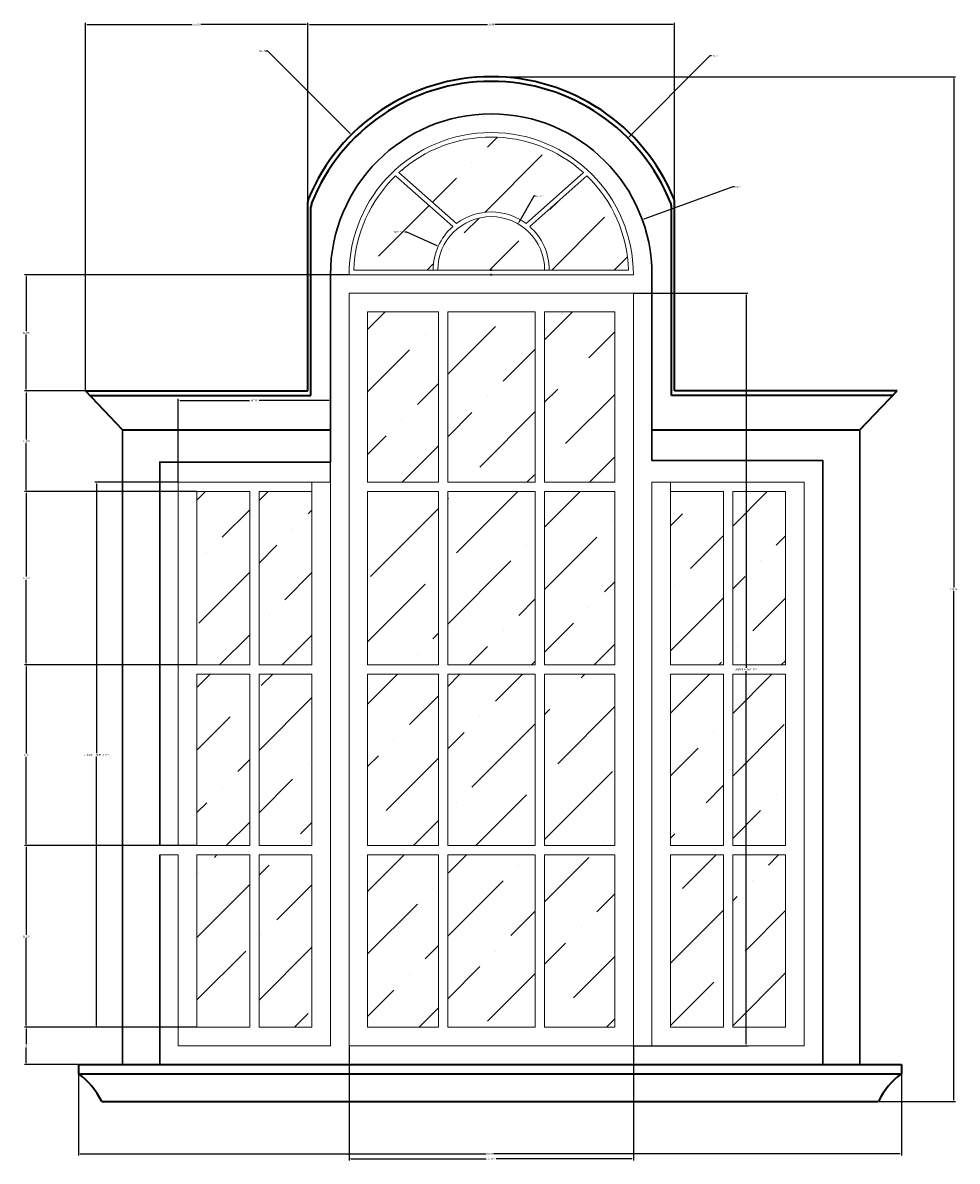
# Model space of a CAD drawing. Units: inches. Extents: x 386 to 708, y 151 to 489.
# Tile 1 of 4: x 386 to 486, y 159 to 281. Entities that reach past the tile are written whole.
import ezdxf

# ---------------------------------------------------------------- set-up
doc = ezdxf.new("R2010")
doc.units = ezdxf.units.IN
doc.header["$MEASUREMENT"] = 0
for name, color, linetype, lineweight in [('A-ANNO-DIMS', 2, 'Continuous', 18), ('A-GLAZ-FRAM', 4, 'Continuous', 30), ('A-GLAZ-PATT', 252, 'Continuous', 13), ('A-GLAZ-SASH', 4, 'Continuous', 18), ('A-GLAZ-SILL', 7, 'Continuous', 35), ('A-GLAZ-TRIM', 7, 'Continuous', 35)]:
    doc.layers.add(name, color=color, linetype=linetype, lineweight=lineweight)
doc.styles.get("Standard").update_dxf_attribs({"font": 'arial.ttf'})
doc.dimstyles.get("Standard").update_dxf_attribs({"dimtxt": 0.18, "dimasz": 0.18, "dimexe": 0.18, "dimexo": 0.0625, "dimgap": 0.09, "dimtad": 0, "dimtih": 1, "dimtoh": 1, "dimdec": 4, "dimzin": 0, "dimdsep": 46, "dimtxsty": 'Standard', "dimcen": 0.09, "dimadec": 0, "dimazin": 0, "dimtfac": 1, "dimtdec": 4, "dimtofl": 0, "dimtmove": 0, "dimatfit": 3, "dimfxl": 1, "dimtolj": 1, "dimtzin": 0, "dimarcsym": 0})

# ---------------------------------------------------------------- blocks, each defined once
blk = doc.blocks.new('WIN-SASH-3X4')
for p, q in [((9.62, 60.63), (9.62, 78.96)), ((10.62, 60.63), (10.62, 78.96)), ((20.04, 60.63), (20.04, 78.96)), ((21.04, 60.63), (21.04, 78.96)), ((2, 60.63), (9.62, 60.63)), ((10.62, 60.63), (20.04, 60.63)), ((21.04, 60.63), (28.6, 60.63)), ((21.04, 60.63), (28.6, 60.63)), ((2, 59.63), (9.62, 59.63)), ((9.62, 40.98), (9.62, 59.63)), ((10.62, 40.98), (10.62, 59.63)), ((10.62, 59.63), (20.04, 59.63)), ((20.04, 40.98), (20.04, 59.63)), ((21.04, 59.63), (28.6, 59.63)), ((21.04, 40.98), (21.04, 59.63)), ((21.04, 59.63), (28.6, 59.63)), ((2, 40.98), (9.62, 40.98)), ((10.62, 40.98), (20.04, 40.98)), ((21.04, 40.98), (28.6, 40.98)), ((21.04, 40.98), (28.6, 40.98)), ((2, 39.98), (9.62, 39.98)), ((9.62, 21.54), (9.62, 39.98)), ((10.62, 21.54), (10.62, 39.98)), ((10.62, 39.98), (20.04, 39.98)), ((20.04, 21.54), (20.04, 39.98)), ((21.04, 39.98), (28.6, 39.98)), ((21.04, 21.54), (21.04, 39.98)), ((21.04, 39.98), (28.6, 39.98)), ((2, 21.54), (9.62, 21.54)), ((10.62, 21.54), (20.04, 21.54)), ((21.04, 21.54), (28.6, 21.54)), ((21.04, 21.54), (28.6, 21.54)), ((2, 20.54), (9.62, 20.54)), ((9.62, 2), (9.62, 20.54)), ((10.62, 2), (10.62, 20.54)), ((10.62, 20.54), (20.04, 20.54)), ((20.04, 2), (20.04, 20.54)), ((21.04, 2), (21.04, 20.54)), ((21.04, 20.54), (28.6, 20.54)), ((21.04, 20.54), (28.6, 20.54))]:
    blk.add_line(p, q)
blk.add_lwpolyline([(30.6, 0), (30.6, 80.96), (0, 80.96), (0, 0)], close=True)
for points in [[(9.62, 78.96), (2, 78.96), (2, 60.63)], [(20.04, 78.96), (10.62, 78.96)], [(28.6, 60.63), (28.6, 78.96), (21.04, 78.96)], [(2, 59.63), (2, 40.98)], [(28.6, 40.98), (28.6, 59.63)], [(2, 39.98), (2, 21.54)], [(28.6, 21.54), (28.6, 39.98)], [(2, 20.54), (2, 2), (9.62, 2)], [(21.04, 2), (28.6, 2), (28.6, 20.54)], [(10.62, 2), (20.04, 2)]]:
    blk.add_lwpolyline(points)
blk = doc.blocks.new('WIN-FANLIGHT-RADIAL')
for p, q in [((11.16, 5.18), (5.01, 10.63)), ((11.55, 5.5), (5.37, 10.98)), ((19.05, 5.5), (25.23, 10.98)), ((19.44, 5.18), (25.6, 10.63))]:
    blk.add_line(p, q)
blk.add_lwpolyline([(30.6, 0), (0, 0, -1)], format="xyb", close=True)
for points in [[(5.37, 10.98, -0.385138), (25.23, 10.98, -0.385138)], [(25.6, 10.63, -0.194348), (30.09, 0.5), (0.51, 0.5, -0.194348), (5.01, 10.63)]]:
    blk.add_lwpolyline(points, format="xyb")
for radius, start, end in [(5.75, 0, 180), (6.25, 53.1161, 126.8839), (6.25, 131.5309, 180), (6.25, 0, 48.4691)]:
    blk.add_arc((15.3, 0.5), radius, start, end)
blk = doc.blocks.new('WIN-SILL-TRIPLE')
for p, q in [((0, 4), (88.59, 4)), ((0, 4), (0, 3)), ((88.59, 4), (88.59, 3)), ((0, 3), (88.59, 3)), ((2.5, 0), (86.09, 0))]:
    blk.add_line(p, q)
blk.add_lwpolyline([(4.75, 0), (84.1, 0)])
for centre, start, end in [((-4.74, -3.48), 25.6893, 53.8074), ((93.33, -3.48), 126.1926, 154.3107)]:
    blk.add_arc(centre, 8.03, start, end)
blk = doc.blocks.new('WIN-LIGHT-GRID-2X3')
for p, q in [((0, 58.63), (7.69, 58.63)), ((2, 57.63), (7.69, 57.63)), ((7.69, 58.63), (16.38, 58.63)), ((7.69, 38.98), (7.69, 57.63)), ((8.69, 38.98), (8.69, 57.63)), ((8.69, 57.63), (14.38, 57.63)), ((2, 38.98), (7.69, 38.98)), ((2, 37.98), (7.69, 37.98)), ((7.69, 19.54), (7.69, 37.98)), ((8.69, 38.98), (14.38, 38.98)), ((8.69, 19.54), (8.69, 37.98)), ((8.69, 37.98), (14.38, 37.98)), ((2, 19.54), (7.69, 19.54)), ((2, 18.54), (7.69, 18.54)), ((7.69, 0), (7.69, 18.54)), ((8.69, 19.54), (14.38, 19.54)), ((8.69, 0), (8.69, 18.54)), ((8.69, 18.54), (14.38, 18.54))]:
    blk.add_line(p, q)
for points in [[(2, 57.63), (2, 38.98)], [(14.38, 38.98), (14.38, 58.63)], [(2, 37.98), (2, 19.54)], [(14.38, 19.54), (14.38, 37.98)], [(2, 18.54), (2, 0), (7.69, 0)], [(8.69, 0), (14.38, 0), (14.38, 18.54)]]:
    blk.add_lwpolyline(points)
blk = doc.blocks.new('*D12')
at = {"layer": 'A-ANNO-DIMS', "color": 0, "lineweight": -2, "transparency": 16777216}
for p, q in [((451.56, 252.21), (463.82, 252.21)), ((463.64, 252.03), (463.64, 211.91)), ((463.64, 171.43), (463.64, 211.55)), ((451.56, 171.25), (463.82, 171.25))]:
    blk.add_line(p, q, dxfattribs=at)
at = {"layer": 'A-ANNO-DIMS', "color": 0, "transparency": 16777216}
for points in [[(463.61, 252.03), (463.67, 252.03), (463.64, 252.21)], [(463.61, 171.43), (463.67, 171.43), (463.64, 171.25)]]:
    blk.add_solid(points, dxfattribs=at)
at = {"layer": 'Defpoints', "color": 0, "transparency": 16777216}
for p in [(451.5, 252.21), (463.64, 252.21), (451.5, 171.25)]:
    blk.add_point(p, dxfattribs=at)
at = {"layer": 'A-ANNO-DIMS', "color": 0, "transparency": 16777216, "insert": (463.64, 211.73), "char_height": 0.18, "attachment_point": 5}
blk.add_mtext('\\A1;CENTRE SASH 81 TYP.', dxfattribs=at)
blk = doc.blocks.new('*D13')
at = {"layer": 'A-ANNO-DIMS', "color": 0, "lineweight": -2, "transparency": 16777216}
for p, q in [((420.9, 171.19), (420.9, 158.93)), ((451.5, 171.19), (451.5, 158.93)), ((421.08, 159.11), (435.67, 159.11)), ((451.32, 159.11), (436.73, 159.11))]:
    blk.add_line(p, q, dxfattribs=at)
at = {"layer": 'A-ANNO-DIMS', "color": 0, "transparency": 16777216}
for points in [[(421.08, 159.14), (421.08, 159.08), (420.9, 159.11)], [(451.32, 159.14), (451.32, 159.08), (451.5, 159.11)]]:
    blk.add_solid(points, dxfattribs=at)
at = {"layer": 'Defpoints', "color": 0, "transparency": 16777216}
for p in [(420.9, 171.25), (451.5, 171.25), (451.5, 159.11)]:
    blk.add_point(p, dxfattribs=at)
at = {"layer": 'A-ANNO-DIMS', "color": 0, "transparency": 16777216, "insert": (436.2, 159.11), "char_height": 0.18, "attachment_point": 5}
blk.add_mtext('\\A1;31 TYP.', dxfattribs=at)
blk = doc.blocks.new('*D20')
at = {"layer": 'A-ANNO-DIMS', "color": 0, "lineweight": -2, "transparency": 16777216}
for p, q in [((402.46, 231.88), (393.55, 231.88)), ((393.73, 231.7), (393.73, 202.75)), ((393.73, 173.43), (393.73, 202.38)), ((402.46, 173.25), (393.55, 173.25))]:
    blk.add_line(p, q, dxfattribs=at)
at = {"layer": 'A-ANNO-DIMS', "color": 0, "transparency": 16777216}
for points in [[(393.7, 231.7), (393.76, 231.7), (393.73, 231.88)], [(393.7, 173.43), (393.76, 173.43), (393.73, 173.25)]]:
    blk.add_solid(points, dxfattribs=at)
at = {"layer": 'Defpoints', "color": 0, "transparency": 16777216}
for p in [(393.73, 231.88), (402.52, 231.88), (402.52, 173.25)]:
    blk.add_point(p, dxfattribs=at)
at = {"layer": 'A-ANNO-DIMS', "color": 0, "transparency": 16777216, "insert": (393.73, 202.57), "char_height": 0.18, "attachment_point": 5}
blk.add_mtext('\\A1;SIDELIGHT GRID 59 TYP.', dxfattribs=at)
blk = doc.blocks.new('*D21')
at = {"layer": 'A-ANNO-DIMS', "color": 0, "lineweight": -2, "transparency": 16777216}
for p, q in [((402.52, 231.94), (402.52, 240.85)), ((402.7, 240.67), (410.19, 240.67)), ((418.72, 240.67), (411.23, 240.67)), ((418.9, 231.94), (418.9, 240.85))]:
    blk.add_line(p, q, dxfattribs=at)
at = {"layer": 'A-ANNO-DIMS', "color": 0, "transparency": 16777216}
for points in [[(402.7, 240.7), (402.7, 240.64), (402.52, 240.67)], [(418.72, 240.7), (418.72, 240.64), (418.9, 240.67)]]:
    blk.add_solid(points, dxfattribs=at)
at = {"layer": 'Defpoints', "color": 0, "transparency": 16777216}
for p in [(418.9, 240.67), (402.52, 231.88), (418.9, 231.88)]:
    blk.add_point(p, dxfattribs=at)
at = {"layer": 'A-ANNO-DIMS', "color": 0, "transparency": 16777216, "insert": (410.71, 240.67), "char_height": 0.18, "attachment_point": 5}
blk.add_mtext('\\A1;16 TYP.', dxfattribs=at)
blk = doc.blocks.new('*D35')
at = {"layer": 'A-ANNO-DIMS', "color": 0, "lineweight": -2, "transparency": 16777216}
for p, q in [((391.77, 169.19), (391.77, 159.45)), ((480.36, 169.19), (480.36, 159.45)), ((391.95, 159.63), (435.67, 159.63)), ((480.18, 159.63), (436.46, 159.63))]:
    blk.add_line(p, q, dxfattribs=at)
at = {"layer": 'A-ANNO-DIMS', "color": 0, "transparency": 16777216}
for points in [[(391.95, 159.66), (391.95, 159.6), (391.77, 159.63)], [(480.18, 159.66), (480.18, 159.6), (480.36, 159.63)]]:
    blk.add_solid(points, dxfattribs=at)
at = {"layer": 'Defpoints', "color": 0, "transparency": 16777216}
for p in [(391.77, 169.25), (480.36, 169.25), (480.36, 159.63)]:
    blk.add_point(p, dxfattribs=at)
at = {"layer": 'A-ANNO-DIMS', "color": 0, "transparency": 16777216, "insert": (436.07, 159.63), "char_height": 0.18, "attachment_point": 5}
blk.add_mtext('\\A1;88.59', dxfattribs=at)
blk = doc.blocks.new('*D36')
at = {"layer": 'A-ANNO-DIMS', "color": 0, "lineweight": -2, "transparency": 16777216}
for p, q in [((436.26, 275.51), (486.16, 275.51)), ((485.98, 275.33), (485.98, 220.56)), ((485.98, 165.43), (485.98, 220.2)), ((477.93, 165.25), (486.16, 165.25))]:
    blk.add_line(p, q, dxfattribs=at)
at = {"layer": 'A-ANNO-DIMS', "color": 0, "transparency": 16777216}
for points in [[(485.95, 275.33), (486.01, 275.33), (485.98, 275.51)], [(485.95, 165.43), (486.01, 165.43), (485.98, 165.25)]]:
    blk.add_solid(points, dxfattribs=at)
at = {"layer": 'Defpoints', "color": 0, "transparency": 16777216}
for p in [(436.2, 275.51), (485.98, 275.51), (477.87, 165.25)]:
    blk.add_point(p, dxfattribs=at)
at = {"layer": 'A-ANNO-DIMS', "color": 0, "transparency": 16777216, "insert": (485.98, 220.38), "char_height": 0.18, "attachment_point": 5}
blk.add_mtext('\\A1;110.26', dxfattribs=at)
blk = doc.blocks.new('*D37')
at = {"layer": 'A-ANNO-DIMS', "color": 0, "lineweight": -2, "transparency": 16777216}
for p, q in [((404.45689, 173.252448), (385.969656, 173.252448)), ((386.149656, 173.072448), (386.149656, 171.432448)), ((386.149656, 169.432448), (386.149656, 171.072448)), ((391.710656, 169.252448), (385.969656, 169.252448))]:
    blk.add_line(p, q, dxfattribs=at)
at = {"layer": 'A-ANNO-DIMS', "color": 0, "transparency": 16777216}
for points in [[(386.119656, 173.072448), (386.179656, 173.072448), (386.149656, 173.252448)], [(386.119656, 169.432448), (386.179656, 169.432448), (386.149656, 169.252448)]]:
    blk.add_solid(points, dxfattribs=at)
at = {"layer": 'Defpoints', "color": 0, "transparency": 16777216}
for p in [(386.149656, 173.252448), (404.51939, 173.252448), (391.773156, 169.252448)]:
    blk.add_point(p, dxfattribs=at)
at = {"layer": 'A-ANNO-DIMS', "color": 0, "transparency": 16777216, "insert": (386.149656, 171.252448), "char_height": 0.18, "attachment_point": 5}
blk.add_mtext('\\A1;4', dxfattribs=at)
blk = doc.blocks.new('*D38')
at = {"layer": 'A-ANNO-DIMS', "color": 0, "lineweight": -2, "transparency": 16777216}
for p, q in [((404.46, 192.79), (385.97, 192.79)), ((386.15, 192.61), (386.15, 183.2)), ((386.15, 173.43), (386.15, 182.84)), ((404.46, 173.25), (385.97, 173.25))]:
    blk.add_line(p, q, dxfattribs=at)
at = {"layer": 'A-ANNO-DIMS', "color": 0, "transparency": 16777216}
for points in [[(386.12, 192.61), (386.18, 192.61), (386.15, 192.79)], [(386.12, 173.43), (386.18, 173.43), (386.15, 173.25)]]:
    blk.add_solid(points, dxfattribs=at)
at = {"layer": 'Defpoints', "color": 0, "transparency": 16777216}
for p in [(386.15, 192.79), (404.52, 192.79), (404.52, 173.25)]:
    blk.add_point(p, dxfattribs=at)
at = {"layer": 'A-ANNO-DIMS', "color": 0, "transparency": 16777216, "insert": (386.15, 183.02), "char_height": 0.18, "attachment_point": 5}
blk.add_mtext('\\A1;19.537', dxfattribs=at)
blk = doc.blocks.new('*D39')
at = {"layer": 'A-ANNO-DIMS', "color": 0, "lineweight": -2, "transparency": 16777216}
for p, q in [((404.46, 212.23), (385.97, 212.23)), ((386.15, 212.05), (386.15, 202.69)), ((386.15, 192.97), (386.15, 202.33)), ((404.46, 192.79), (385.97, 192.79))]:
    blk.add_line(p, q, dxfattribs=at)
at = {"layer": 'A-ANNO-DIMS', "color": 0, "transparency": 16777216}
for points in [[(386.12, 212.05), (386.18, 212.05), (386.15, 212.23)], [(386.12, 192.97), (386.18, 192.97), (386.15, 192.79)]]:
    blk.add_solid(points, dxfattribs=at)
at = {"layer": 'Defpoints', "color": 0, "transparency": 16777216}
for p in [(386.15, 212.23), (404.52, 212.23), (404.52, 192.79)]:
    blk.add_point(p, dxfattribs=at)
at = {"layer": 'A-ANNO-DIMS', "color": 0, "transparency": 16777216, "insert": (386.15, 202.51), "char_height": 0.18, "attachment_point": 5}
blk.add_mtext('\\A1;19.44', dxfattribs=at)
blk = doc.blocks.new('*D40')
at = {"layer": 'A-ANNO-DIMS', "color": 0, "lineweight": -2, "transparency": 16777216}
for p, q in [((404.46, 230.88), (385.97, 230.88)), ((386.15, 230.7), (386.15, 221.74)), ((386.15, 212.41), (386.15, 221.37)), ((404.46, 212.23), (385.97, 212.23))]:
    blk.add_line(p, q, dxfattribs=at)
at = {"layer": 'A-ANNO-DIMS', "color": 0, "transparency": 16777216}
for points in [[(386.12, 230.7), (386.18, 230.7), (386.15, 230.88)], [(386.12, 212.41), (386.18, 212.41), (386.15, 212.23)]]:
    blk.add_solid(points, dxfattribs=at)
at = {"layer": 'Defpoints', "color": 0, "transparency": 16777216}
for p in [(386.15, 230.88), (404.52, 230.88), (404.52, 212.23)]:
    blk.add_point(p, dxfattribs=at)
at = {"layer": 'A-ANNO-DIMS', "color": 0, "transparency": 16777216, "insert": (386.15, 221.55), "char_height": 0.18, "attachment_point": 5}
blk.add_mtext('\\A1;18.648', dxfattribs=at)
blk = doc.blocks.new('*D41')
at = {"layer": 'A-ANNO-DIMS', "color": 0, "lineweight": -2, "transparency": 16777216}
for p, q in [((392.46, 241.7), (385.97, 241.7)), ((386.15, 241.52), (386.15, 236.47)), ((386.15, 231.06), (386.15, 236.11)), ((404.46, 230.88), (385.97, 230.88))]:
    blk.add_line(p, q, dxfattribs=at)
at = {"layer": 'A-ANNO-DIMS', "color": 0, "transparency": 16777216}
for points in [[(386.12, 241.52), (386.18, 241.52), (386.15, 241.7)], [(386.12, 231.06), (386.18, 231.06), (386.15, 230.88)]]:
    blk.add_solid(points, dxfattribs=at)
at = {"layer": 'Defpoints', "color": 0, "transparency": 16777216}
for p in [(386.15, 241.7), (392.52, 241.7), (404.52, 230.88)]:
    blk.add_point(p, dxfattribs=at)
at = {"layer": 'A-ANNO-DIMS', "color": 0, "transparency": 16777216, "insert": (386.15, 236.29), "char_height": 0.18, "attachment_point": 5}
blk.add_mtext('\\A1;10.825', dxfattribs=at)
blk = doc.blocks.new('*D42')
at = {"layer": 'A-ANNO-DIMS', "color": 0, "lineweight": -2, "transparency": 16777216}
for p, q in [((420.83, 254.21), (385.97, 254.21)), ((386.15, 254.03), (386.15, 248.14)), ((386.15, 241.88), (386.15, 247.77)), ((392.46, 241.7), (385.97, 241.7))]:
    blk.add_line(p, q, dxfattribs=at)
at = {"layer": 'A-ANNO-DIMS', "color": 0, "transparency": 16777216}
for points in [[(386.12, 254.03), (386.18, 254.03), (386.15, 254.21)], [(386.12, 241.88), (386.18, 241.88), (386.15, 241.7)]]:
    blk.add_solid(points, dxfattribs=at)
at = {"layer": 'Defpoints', "color": 0, "transparency": 16777216}
for p in [(386.15, 254.21), (420.9, 254.21), (392.52, 241.7)]:
    blk.add_point(p, dxfattribs=at)
at = {"layer": 'A-ANNO-DIMS', "color": 0, "transparency": 16777216, "insert": (386.15, 247.96), "char_height": 0.18, "attachment_point": 5}
blk.add_mtext('\\A1;12.505', dxfattribs=at)
blk = doc.blocks.new('*D43')
at = {"layer": 'A-ANNO-DIMS', "color": 0, "lineweight": -2, "transparency": 16777216}
for p, q in [((416.46, 241.77), (416.46, 281.31)), ((416.64, 281.13), (435.8, 281.13)), ((455.76, 281.13), (436.59, 281.13)), ((455.94, 241.77), (455.94, 281.31))]:
    blk.add_line(p, q, dxfattribs=at)
at = {"layer": 'A-ANNO-DIMS', "color": 0, "transparency": 16777216}
for points in [[(416.64, 281.16), (416.64, 281.1), (416.46, 281.13)], [(455.76, 281.16), (455.76, 281.1), (455.94, 281.13)]]:
    blk.add_solid(points, dxfattribs=at)
at = {"layer": 'Defpoints', "color": 0, "transparency": 16777216}
for p in [(455.94, 281.13), (416.46, 241.7), (455.94, 241.7)]:
    blk.add_point(p, dxfattribs=at)
at = {"layer": 'A-ANNO-DIMS', "color": 0, "transparency": 16777216, "insert": (436.2, 281.13), "char_height": 0.18, "attachment_point": 5}
blk.add_mtext('\\A1;39.48', dxfattribs=at)
blk = doc.blocks.new('*D44')
at = {"layer": 'A-ANNO-DIMS', "color": 0, "lineweight": -2, "transparency": 16777216}
for p, q in [((392.52, 241.77), (392.52, 281.31)), ((392.7, 281.13), (404.02, 281.13)), ((416.28, 281.13), (404.95, 281.13)), ((416.46, 241.77), (416.46, 281.31))]:
    blk.add_line(p, q, dxfattribs=at)
at = {"layer": 'A-ANNO-DIMS', "color": 0, "transparency": 16777216}
for points in [[(392.7, 281.16), (392.7, 281.1), (392.52, 281.13)], [(416.28, 281.16), (416.28, 281.1), (416.46, 281.13)]]:
    blk.add_solid(points, dxfattribs=at)
at = {"layer": 'Defpoints', "color": 0, "transparency": 16777216}
for p in [(416.46, 281.13), (392.52, 241.7), (416.46, 241.7)]:
    blk.add_point(p, dxfattribs=at)
at = {"layer": 'A-ANNO-DIMS', "color": 0, "transparency": 16777216, "insert": (404.49, 281.13), "char_height": 0.18, "attachment_point": 5}
blk.add_mtext('\\A1;23.937', dxfattribs=at)
blk = doc.blocks.new('*D83')
at = {"layer": 'A-ANNO-DIMS', "color": 0, "lineweight": -2, "transparency": 16777216}
for p, q in [((411.92, 278.31), (412.1, 278.31)), ((412.1, 278.31), (421.01, 269.4)), ((436.11, 254.21), (436.29, 254.21)), ((436.2, 254.12), (436.2, 254.3))]:
    blk.add_line(p, q, dxfattribs=at)
at = {"layer": 'A-ANNO-DIMS', "color": 0, "transparency": 16777216}
blk.add_solid([(421.03, 269.42), (420.99, 269.38), (421.14, 269.27)], dxfattribs=at)
at = {"layer": 'Defpoints', "color": 0, "transparency": 16777216}
for p in [(421.14, 269.27), (436.2, 254.21)]:
    blk.add_point(p, dxfattribs=at)
at = {"layer": 'A-ANNO-DIMS', "color": 0, "transparency": 16777216, "insert": (411.51, 278.31), "char_height": 0.18, "attachment_point": 5}
blk.add_mtext('\\A1;R21.3', dxfattribs=at)
blk = doc.blocks.new('*D84')
at = {"layer": 'A-ANNO-DIMS', "color": 0, "lineweight": -2, "transparency": 16777216}
for p, q in [((459.73, 277.74), (451.03, 269.04)), ((459.91, 277.74), (459.73, 277.74)), ((436.11, 254.21), (436.29, 254.21)), ((436.2, 254.12), (436.2, 254.3))]:
    blk.add_line(p, q, dxfattribs=at)
at = {"layer": 'A-ANNO-DIMS', "color": 0, "transparency": 16777216}
blk.add_solid([(451.01, 269.07), (451.06, 269.02), (450.91, 268.92)], dxfattribs=at)
at = {"layer": 'Defpoints', "color": 0, "transparency": 16777216}
for p in [(450.91, 268.92), (436.2, 254.21)]:
    blk.add_point(p, dxfattribs=at)
at = {"layer": 'A-ANNO-DIMS', "color": 0, "transparency": 16777216, "insert": (460.32, 277.74), "char_height": 0.18, "attachment_point": 5}
blk.add_mtext('\\A1;R20.8', dxfattribs=at)
blk = doc.blocks.new('*D85')
at = {"layer": 'A-ANNO-DIMS', "color": 0, "lineweight": -2, "transparency": 16777216}
for p, q in [((462.21, 263.68), (452.63, 260.19)), ((462.39, 263.68), (462.21, 263.68)), ((436.11, 254.21), (436.29, 254.21)), ((436.2, 254.12), (436.2, 254.3))]:
    blk.add_line(p, q, dxfattribs=at)
at = {"layer": 'A-ANNO-DIMS', "color": 0, "transparency": 16777216}
blk.add_solid([(452.62, 260.22), (452.64, 260.16), (452.46, 260.13)], dxfattribs=at)
at = {"layer": 'Defpoints', "color": 0, "transparency": 16777216}
for p in [(452.46, 260.13), (436.2, 254.21)]:
    blk.add_point(p, dxfattribs=at)
at = {"layer": 'A-ANNO-DIMS', "color": 0, "transparency": 16777216, "insert": (462.8, 263.68), "char_height": 0.18, "attachment_point": 5}
blk.add_mtext('\\A1;R17.3', dxfattribs=at)
blk = doc.blocks.new('*D86')
at = {"layer": 'A-ANNO-DIMS', "color": 0, "lineweight": -2, "transparency": 16777216}
for p, q in [((426.9, 258.81), (427.08, 258.81)), ((427.08, 258.81), (430.34, 257.35)), ((436.2, 254.62), (436.2, 254.8)), ((436.11, 254.71), (436.29, 254.71))]:
    blk.add_line(p, q, dxfattribs=at)
at = {"layer": 'A-ANNO-DIMS', "color": 0, "transparency": 16777216}
blk.add_solid([(430.35, 257.37), (430.33, 257.32), (430.5, 257.27)], dxfattribs=at)
at = {"layer": 'Defpoints', "color": 0, "transparency": 16777216}
for p in [(430.5, 257.27), (436.2, 254.71)]:
    blk.add_point(p, dxfattribs=at)
at = {"layer": 'A-ANNO-DIMS', "color": 0, "transparency": 16777216, "insert": (426.23, 258.81), "char_height": 0.18, "attachment_point": 5}
blk.add_mtext('\\A1;3X R6.247', dxfattribs=at)
blk = doc.blocks.new('*D87')
at = {"layer": 'A-ANNO-DIMS', "color": 0, "lineweight": -2, "transparency": 16777216}
for p, q in [((440.8, 262.67), (439.16, 259.84)), ((440.98, 262.67), (440.8, 262.67)), ((436.2, 254.62), (436.2, 254.8)), ((436.11, 254.71), (436.29, 254.71))]:
    blk.add_line(p, q, dxfattribs=at)
at = {"layer": 'A-ANNO-DIMS', "color": 0, "transparency": 16777216}
blk.add_solid([(439.14, 259.86), (439.19, 259.83), (439.07, 259.69)], dxfattribs=at)
at = {"layer": 'Defpoints', "color": 0, "transparency": 16777216}
for p in [(439.07, 259.69), (436.2, 254.71)]:
    blk.add_point(p, dxfattribs=at)
at = {"layer": 'A-ANNO-DIMS', "color": 0, "transparency": 16777216, "insert": (441.46, 262.67), "char_height": 0.18, "attachment_point": 5}
blk.add_mtext('\\A1;R5.747', dxfattribs=at)

msp = doc.modelspace()

# ---------------------------------------------------------------- hatches: boundary and pattern name
at = {"layer": 'A-GLAZ-PATT'}
h = msp.add_hatch(dxfattribs=at)
h.set_pattern_fill('ANSI36', color=256, scale=38)
h.set_pattern_definition([(45, (0, -201.4496), (2.519068, 9.236582), [11.875, -2.375, 0, -2.375])])
h.paths.add_polyline_path([(432.0564, 259.3848, 0.21469693), (429.9512, 254.7081), (430.4512, 254.7081, -1), (441.9457, 254.7081), (442.4457, 254.7081, 0.21469693), (440.3405, 259.3848), (446.4934, 264.8423, -0.19434814), (450.9912, 254.7081), (421.4058, 254.7081, -0.19434814), (425.9035, 264.8423)])
h.paths.add_polyline_path([(446.1268, 265.1855, 0.38513823), (426.2702, 265.1855), (432.4489, 259.705, -0.33346908), (439.948, 259.705)])
h.paths.add_polyline_path([(449.4996, 250.2081), (441.9385, 250.2081), (441.9385, 231.878), (449.4996, 231.878)])
h.paths.add_polyline_path([(440.9385, 250.2081), (431.5153, 250.2081), (431.5153, 231.878), (440.9385, 231.878)])
h.paths.add_polyline_path([(430.5153, 250.2081), (422.8973, 250.2081), (422.8973, 231.878), (430.5153, 231.878)])
h.paths.add_polyline_path([(410.2084, 230.878), (404.5194, 230.878), (404.5194, 212.2303), (410.2084, 212.2303)])
h.paths.add_polyline_path([(416.8973, 230.878), (411.2084, 230.878), (411.2084, 212.2303), (416.8973, 212.2303)])
h.paths.add_polyline_path([(430.5153, 230.878), (422.8973, 230.878), (422.8973, 212.2303), (430.5153, 212.2303)])
h.paths.add_polyline_path([(440.9385, 230.878), (431.5153, 230.878), (431.5153, 212.2303), (440.9385, 212.2303)])
h.paths.add_polyline_path([(449.4996, 230.878), (441.9385, 230.878), (441.9385, 212.2303), (449.4996, 212.2303)])
h.paths.add_polyline_path([(461.1886, 230.878), (455.4996, 230.878), (455.4996, 212.2303), (461.1886, 212.2303)])
h.paths.add_polyline_path([(467.8775, 230.878), (462.1886, 230.878), (462.1886, 212.2303), (467.8775, 212.2303)])
h.paths.add_polyline_path([(467.8775, 211.2303), (462.1886, 211.2303), (462.1886, 192.7894), (467.8775, 192.7894)])
h.paths.add_polyline_path([(461.1886, 211.2303), (455.4996, 211.2303), (455.4996, 192.7894), (461.1886, 192.7894)])
h.paths.add_polyline_path([(449.4996, 211.2303), (441.9385, 211.2303), (441.9385, 192.7894), (449.4996, 192.7894)])
h.paths.add_polyline_path([(440.9385, 211.2303), (431.5153, 211.2303), (431.5153, 192.7894), (440.9385, 192.7894)])
h.paths.add_polyline_path([(430.5153, 211.2303), (422.8973, 211.2303), (422.8973, 192.7894), (430.5153, 192.7894)])
h.paths.add_polyline_path([(416.8973, 211.2303), (411.2084, 211.2303), (411.2084, 192.7894), (416.8973, 192.7894)])
h.paths.add_polyline_path([(410.2084, 211.2303), (404.5194, 211.2303), (404.5194, 192.7894), (410.2084, 192.7894)])
h.paths.add_polyline_path([(410.2084, 191.7894), (404.5194, 191.7894), (404.5194, 173.2524), (410.2084, 173.2524)])
h.paths.add_polyline_path([(416.8973, 191.7894), (411.2084, 191.7894), (411.2084, 173.2524), (416.8973, 173.2524)])
h.paths.add_polyline_path([(430.5153, 191.7894), (422.8973, 191.7894), (422.8973, 173.2524), (430.5153, 173.2524)])
h.paths.add_polyline_path([(440.9385, 191.7894), (431.5153, 191.7894), (431.5153, 173.2524), (440.9385, 173.2524)])
h.paths.add_polyline_path([(449.4996, 191.7894), (441.9385, 191.7894), (441.9385, 173.2524), (449.4996, 173.2524)])
h.paths.add_polyline_path([(461.1886, 191.7894), (455.4996, 191.7894), (455.4996, 173.2524), (461.1886, 173.2524)])
h.paths.add_polyline_path([(467.8775, 191.7894), (462.1886, 191.7894), (462.1886, 173.2524), (467.8775, 173.2524)])

# ---------------------------------------------------------------- linework, layer by layer
at = {"layer": 'A-GLAZ-FRAM'}
for points in [[(418.8973, 234.0458), (418.8973, 254.2081)], [(453.4996, 254.2081), (453.4996, 234.2336)], [(396.5194, 237.5069), (396.5194, 169.2524)], [(475.8775, 169.2524), (475.8775, 237.5069)], [(400.5194, 191.7894), (400.5194, 169.2524), (471.8775, 169.2524), (471.8775, 234.2336), (453.4996, 234.2336)], [(418.8973, 234.0458), (400.5194, 234.0458), (400.5194, 192.7894)]]:
    msp.add_lwpolyline(points, dxfattribs=at)
msp.add_arc((436.1985, 254.2081), 17.3011, 0, 180, dxfattribs=at)
at = {"layer": 'A-GLAZ-SASH'}
for p, q in [((400.5194, 192.7894), (402.5194, 192.7894)), ((400.5194, 191.7894), (402.5194, 191.7894))]:
    msp.add_line(p, q, dxfattribs=at)
for points in [[(402.5194, 191.7894), (402.5194, 171.2524), (418.8973, 171.2524), (418.8973, 231.878)], [(402.5194, 231.878), (402.5194, 192.7894)], [(453.4996, 231.878), (453.4996, 171.2524), (469.8775, 171.2524), (469.8775, 231.878)]]:
    msp.add_lwpolyline(points, dxfattribs=at)
at = {"layer": 'A-GLAZ-TRIM'}
for p, q in [((416.4567, 241.7029), (416.4567, 262.0107)), ((416.7965, 241.2029), (416.7965, 261.5192)), ((455.6005, 241.2029), (455.6005, 261.5192)), ((455.9403, 241.7029), (455.9403, 262.0107)), ((392.5194, 241.7029), (416.4567, 241.7029)), ((396.5194, 237.5069), (392.5194, 241.7029)), ((479.8775, 241.7029), (455.9403, 241.7029)), ((475.8775, 237.5069), (479.8775, 241.7029)), ((393.0194, 241.2029), (416.7965, 241.2029)), ((479.3775, 241.2029), (455.6005, 241.2029)), ((396.5194, 237.5069), (418.8973, 237.5069)), ((453.4996, 237.5069), (475.8775, 237.5069))]:
    msp.add_line(p, q, dxfattribs=at)
for centre, radius, start, end in [((436.1985, 254.2081), 21.3011, 22.603102, 157.396898), ((436.1985, 254.2081), 20.8011, 21.667803, 158.332197), ((417.4567, 262.0107), 1, 157.396898, 180), ((417.4567, 262.0107), 1, 157.396898, 180), ((454.9403, 262.0107), 1, 0, 22.603102), ((417.7965, 261.5192), 1, 158.332197, 180), ((454.6005, 261.5192), 1, 0, 21.667803)]:
    msp.add_arc(centre, radius, start, end, dxfattribs=at)

# ---------------------------------------------------------------- block references
at = {"layer": 'A-GLAZ-SASH'}
for name, p in [('WIN-FANLIGHT-RADIAL', (420.897, 254.2084)), ('WIN-SASH-3X4', (420.897, 171.2524)), ('WIN-LIGHT-GRID-2X3', (402.519, 173.252))]:
    msp.add_blockref(name, p, dxfattribs=at)
at = {"layer": 'A-GLAZ-SASH', "extrusion": (0, 0, -1), "zscale": -1}
msp.add_blockref('WIN-LIGHT-GRID-2X3', (-469.8779, 173.252), dxfattribs=at)
at = {"layer": 'A-GLAZ-SILL'}
msp.add_blockref('WIN-SILL-TRIPLE', (391.773, 165.2524), dxfattribs=at)

# ---------------------------------------------------------------- dimensions: what is measured, and where the dimension line sits
at = {"layer": 'A-ANNO-DIMS'}
for base, p1, p2, override, picture, middle in [((416.4567, 281.1327), (392.5194, 241.7029), (416.4567, 241.7029), {"dimdec": 3, "dimlfac": 1, "dimrnd": 0, "dimzin": 0, "dimdsep": 46, "dimlunit": 2}, '*D44', (404.488, 281.1327)), ((455.9403, 281.1327), (416.4567, 241.7029), (455.9403, 241.7029), {"dimdec": 2, "dimlfac": 1, "dimrnd": 0, "dimzin": 0, "dimdsep": 46, "dimlunit": 2}, '*D43', (436.1985, 281.1327)), ((480.3605, 159.6289), (391.7732, 169.2524), (480.3605, 169.2524), {"dimdec": 2, "dimlfac": 1, "dimrnd": 0, "dimzin": 0, "dimdsep": 46, "dimlunit": 2}, '*D35', (436.0669, 159.6289))]:
    dim = msp.add_linear_dim(base=base, p1=p1, p2=p2, dimstyle='Standard', override=override, dxfattribs=at)
    dim.commit()
    dim.dimension.update_dxf_attribs({"geometry": picture, "text_midpoint": middle})
for center, mpoint, override, picture, middle in [((436.1985, 254.2081), (421.136, 269.27), {"dimdec": 1, "dimlfac": 1, "dimrnd": 0, "dimzin": 0, "dimdsep": 46, "dimlunit": 2}, '*D83', (411.5086, 278.3071)), ((436.1985, 254.2081), (450.9069, 268.9169), {"dimdec": 1, "dimlfac": 1, "dimrnd": 0, "dimzin": 0, "dimdsep": 46, "dimlunit": 2}, '*D84', (460.3221, 277.7422)), ((436.1985, 254.2081), (452.4562, 260.1254), {"dimdec": 1, "dimlfac": 1, "dimrnd": 0, "dimzin": 0, "dimdsep": 46, "dimlunit": 2}, '*D85', (462.8008, 263.6759)), ((436.1985, 254.7081), (439.0722, 259.6853), {"dimdec": 3, "dimlfac": 1, "dimrnd": 0, "dimzin": 0, "dimdsep": 46, "dimlunit": 2}, '*D87', (441.4562, 262.6716))]:
    dim = msp.add_radius_dim(center=center, mpoint=mpoint, dimstyle='Standard', override=override, dxfattribs=at)
    dim.commit()
    dim.dimension.update_dxf_attribs({"geometry": picture, "text_midpoint": middle, "dimtype": 164})
for base, p1, p2, override, picture, middle in [((485.9841, 275.5092), (477.8656, 165.2524), (436.1985, 275.5092), {"dimdec": 2, "dimlfac": 1, "dimrnd": 0, "dimzin": 0, "dimdsep": 46, "dimlunit": 2}, '*D36', (485.9841, 220.3808)), ((386.1497, 254.2081), (392.5194, 241.7029), (420.8973, 254.2081), {"dimdec": 3, "dimlfac": 1, "dimrnd": 0, "dimzin": 0, "dimdsep": 46, "dimlunit": 2}, '*D42', (386.1497, 247.9555)), ((386.1497, 241.7029), (404.5194, 230.878), (392.5194, 241.7029), {"dimdec": 3, "dimlfac": 1, "dimrnd": 0, "dimzin": 0, "dimdsep": 46, "dimlunit": 2}, '*D41', (386.1497, 236.2904)), ((386.1497, 230.878), (404.5194, 212.2303), (404.5194, 230.878), {"dimdec": 3, "dimlfac": 1, "dimrnd": 0, "dimzin": 0, "dimdsep": 46, "dimlunit": 2}, '*D40', (386.1497, 221.5541)), ((386.1497, 212.2303), (404.5194, 192.7894), (404.5194, 212.2303), {"dimdec": 2, "dimlfac": 1, "dimrnd": 0, "dimzin": 0, "dimdsep": 46, "dimlunit": 2}, '*D39', (386.1497, 202.5099)), ((386.1497, 192.7894), (404.5194, 173.2524), (404.5194, 192.7894), {"dimdec": 3, "dimlfac": 1, "dimrnd": 0, "dimzin": 0, "dimdsep": 46, "dimlunit": 2}, '*D38', (386.1497, 183.0209)), ((386.1497, 173.2524), (391.7732, 169.2524), (404.5194, 173.2524), {"dimdec": 0, "dimlfac": 1, "dimrnd": 0, "dimzin": 0, "dimdsep": 46, "dimlunit": 2}, '*D37', (386.1497, 171.2524))]:
    dim = msp.add_linear_dim(base=base, p1=p1, p2=p2, angle=90, dimstyle='Standard', override=override, dxfattribs=at)
    dim.commit()
    dim.dimension.update_dxf_attribs({"geometry": picture, "text_midpoint": middle})
dim = msp.add_radius_dim(center=(436.1985, 254.7081), mpoint=(430.5017, 257.2722), text='3X <>', dimstyle='Standard', override={"dimdec": 3, "dimlfac": 1, "dimrnd": 0, "dimzin": 0, "dimdsep": 46, "dimlunit": 2}, dxfattribs=at)
dim.commit()
dim.dimension.update_dxf_attribs({"geometry": '*D86', "text_midpoint": (426.2304, 258.8106), "dimtype": 164})
for base, p1, p2, text, picture, middle in [((463.643, 252.2081), (451.4996, 171.2524), (451.4996, 252.2081), 'CENTRE SASH <> TYP.', '*D12', (463.643, 211.7303)), ((393.7256, 231.878), (402.5194, 173.2524), (402.5194, 231.878), 'SIDELIGHT GRID <> TYP.', '*D20', (393.7256, 202.5652))]:
    dim = msp.add_linear_dim(base=base, p1=p1, p2=p2, angle=90, text=text, dimstyle='Standard', override={"dimdec": 0, "dimlfac": 1, "dimrnd": 0, "dimzin": 0, "dimdsep": 46, "dimlunit": 2}, dxfattribs=at)
    dim.commit()
    dim.dimension.update_dxf_attribs({"geometry": picture, "text_midpoint": middle})
for base, p1, p2, picture, middle in [((418.8973, 240.6718), (402.5194, 231.878), (418.8973, 231.878), '*D21', (410.7084, 240.6718)), ((451.4996, 159.1091), (420.8973, 171.2524), (451.4996, 171.2524), '*D13', (436.1985, 159.1091))]:
    dim = msp.add_linear_dim(base=base, p1=p1, p2=p2, text='<> TYP.', dimstyle='Standard', override={"dimdec": 0, "dimlfac": 1, "dimrnd": 0, "dimzin": 0, "dimdsep": 46, "dimlunit": 2}, dxfattribs=at)
    dim.commit()
    dim.dimension.update_dxf_attribs({"geometry": picture, "text_midpoint": middle})

doc.saveas('drawing.dxf')
